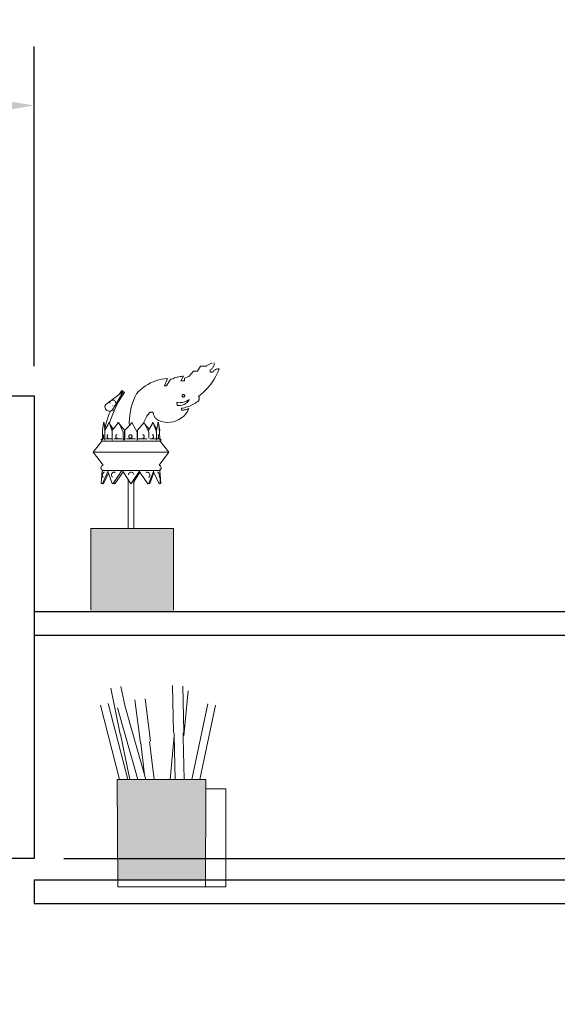
# Model space of a CAD drawing. Units: millimetres. Extents: x 7894 to 8038, y 6851 to 6951.
# Tile 8 of 49: x 7963 to 7975, y 6871 to 6892. Entities that reach past the tile are written whole.
import ezdxf

# ---------------------------------------------------------------- set-up
doc = ezdxf.new("R2010")
doc.units = ezdxf.units.MM
for name, color, linetype, lineweight in [('A-ANNO-DIMS', 2, 'Continuous', 18), ('A-FURN-ACCS', 8, 'Continuous', 13), ('A-FURN-CASE', 7, 'Continuous', 30), ('A-FURN-SHLF', 7, 'Continuous', 30)]:
    doc.layers.add(name, color=color, linetype=linetype, lineweight=lineweight)
doc.layers.add('A-FURN-ACCS-PATT', color=116, linetype='Continuous', lineweight=9, true_color=0x136734)
doc.styles.get("Standard").update_dxf_attribs({"font": 'arial.ttf'})
doc.dimstyles.new('ISO-25', dxfattribs={"dimtxt": 1, "dimasz": 1, "dimexe": 1.25, "dimexo": 0.625, "dimtad": 1, "dimdec": 0, "dimlunit": 4, "dimtxsty": 'Standard', "dimcen": 2.5, "dimclrt": 1, "dimadec": 0, "dimazin": 0, "dimtfac": 1, "dimtdec": 0, "dimtmove": 0, "dimatfit": 3, "dimfxl": 1, "dimarcsym": 0})

# ---------------------------------------------------------------- blocks, each defined once
blk = doc.blocks.new('DISPLAY-LEAF-FINIAL')
for p, q in [((2.209, 3.334), (2.276, 3.441)), ((2.276, 3.441), (2.398, 3.441)), ((2.398, 3.441), (2.409, 3.452)), ((2.409, 3.452), (2.421, 3.461)), ((2.421, 3.461), (2.434, 3.47)), ((2.434, 3.47), (2.447, 3.478)), ((2.447, 3.478), (2.461, 3.485)), ((2.461, 3.485), (2.475, 3.491)), ((2.475, 3.491), (2.489, 3.496)), ((2.493, 3.371), (2.48, 3.364)), ((2.48, 3.364), (2.48, 3.316)), ((2.489, 3.496), (2.504, 3.501)), ((2.505, 3.379), (2.493, 3.371)), ((2.504, 3.501), (2.519, 3.504)), ((2.516, 3.389), (2.505, 3.379)), ((2.527, 3.4), (2.516, 3.389)), ((2.536, 3.411), (2.527, 3.4)), ((2.544, 3.424), (2.536, 3.411)), ((2.54, 3.327), (2.549, 3.338)), ((2.551, 3.437), (2.544, 3.424)), ((2.549, 3.338), (2.558, 3.347)), ((2.556, 3.45), (2.551, 3.437)), ((2.56, 3.465), (2.556, 3.45)), ((2.558, 3.347), (2.569, 3.356)), ((2.563, 3.479), (2.56, 3.465)), ((2.565, 3.494), (2.563, 3.479)), ((2.565, 3.508), (2.565, 3.494)), ((2.569, 3.356), (2.58, 3.363)), ((2.58, 3.363), (2.592, 3.37)), ((2.592, 3.37), (2.604, 3.375)), ((2.604, 3.375), (2.617, 3.379)), ((2.617, 3.379), (2.63, 3.382)), ((2.63, 3.382), (2.643, 3.383)), ((2.643, 3.383), (2.657, 3.383)), ((2.67, 3.382), (2.646, 3.325)), ((2.657, 3.383), (2.67, 3.382)), ((1.27, 3.111), (1.328, 3.133)), ((1.328, 3.133), (1.388, 3.15)), ((1.388, 3.15), (1.449, 3.164)), ((1.449, 3.164), (1.51, 3.173)), ((1.51, 3.173), (1.572, 3.179)), ((1.572, 3.179), (1.511, 3.024)), ((1.55, 3.024), (1.632, 3.152)), ((1.632, 3.152), (1.654, 3.163)), ((1.654, 3.163), (1.676, 3.173)), ((1.676, 3.173), (1.699, 3.182)), ((1.699, 3.182), (1.722, 3.191)), ((1.722, 3.191), (1.745, 3.198)), ((1.745, 3.198), (1.769, 3.205)), ((1.769, 3.205), (1.793, 3.211)), ((1.793, 3.211), (1.817, 3.216)), ((1.817, 3.216), (1.841, 3.22)), ((1.841, 3.22), (1.865, 3.223)), ((1.914, 3.227), (1.854, 3.133)), ((1.854, 3.133), (1.934, 3.133)), ((1.865, 3.223), (1.889, 3.226)), ((1.889, 3.226), (1.914, 3.227)), ((1.934, 3.185), (2.023, 3.221)), ((1.934, 3.133), (1.934, 3.185)), ((2.023, 3.221), (2.127, 3.334)), ((2.127, 3.334), (2.209, 3.334)), ((2.48, 3.316), (2.533, 3.316)), ((2.56, 3.163), (2.527, 3.112)), ((2.533, 3.316), (2.54, 3.327)), ((2.591, 3.216), (2.56, 3.163)), ((2.62, 3.27), (2.591, 3.216)), ((2.646, 3.325), (2.62, 3.27)), ((0.605, 2.924), (0.547, 2.84)), ((0.634, 2.905), (0.605, 2.924)), ((0.962, 2.903), (1.007, 2.946)), ((1.007, 2.946), (1.055, 2.986)), ((1.055, 2.986), (1.105, 3.023)), ((1.105, 3.023), (1.158, 3.056)), ((1.158, 3.056), (1.213, 3.085)), ((1.213, 3.085), (1.27, 3.111)), ((1.511, 3.024), (1.55, 3.024)), ((2.371, 2.923), (2.327, 2.88)), ((2.413, 2.967), (2.371, 2.923)), ((2.453, 3.014), (2.413, 2.967)), ((2.491, 3.062), (2.453, 3.014)), ((2.527, 3.112), (2.491, 3.062)), ((0.379, 2.713), (0.264, 2.627)), ((0.367, 2.703), (0.379, 2.713)), ((0.547, 2.84), (0.379, 2.713)), ((0.379, 2.713), (0.393, 2.72)), ((0.393, 2.72), (0.409, 2.723)), ((0.409, 2.723), (0.425, 2.722)), ((0.425, 2.722), (0.44, 2.718)), ((0.44, 2.718), (0.453, 2.709)), ((0.634, 2.9), (0.463, 2.609)), ((0.541, 2.696), (0.599, 2.791)), ((0.634, 2.905), (0.547, 2.84)), ((0.599, 2.791), (0.663, 2.885)), ((0.634, 2.9), (0.634, 2.905)), ((0.663, 2.885), (0.634, 2.905)), ((0.853, 2.713), (0.826, 2.638)), ((0.884, 2.786), (0.853, 2.713)), ((0.92, 2.857), (0.884, 2.786)), ((0.92, 2.857), (0.962, 2.903)), ((1.883, 2.817), (1.885, 2.824)), ((1.883, 2.81), (1.883, 2.817)), ((1.885, 2.803), (1.883, 2.81)), ((1.885, 2.824), (1.889, 2.831)), ((1.888, 2.797), (1.885, 2.803)), ((1.894, 2.791), (1.888, 2.797)), ((1.889, 2.831), (1.894, 2.836)), ((1.894, 2.836), (1.9, 2.839)), ((1.9, 2.788), (1.894, 2.791)), ((1.9, 2.839), (1.907, 2.841)), ((1.907, 2.786), (1.9, 2.788)), ((1.907, 2.841), (1.914, 2.841)), ((1.914, 2.786), (1.907, 2.786)), ((1.914, 2.841), (1.921, 2.839)), ((1.921, 2.788), (1.914, 2.786)), ((1.921, 2.839), (1.928, 2.836)), ((1.928, 2.791), (1.921, 2.788)), ((1.928, 2.836), (1.933, 2.83)), ((1.933, 2.796), (1.928, 2.791)), ((1.933, 2.83), (1.937, 2.824)), ((1.936, 2.803), (1.933, 2.796)), ((1.938, 2.81), (1.936, 2.803)), ((1.937, 2.824), (1.938, 2.817)), ((1.938, 2.817), (1.938, 2.81)), ((2.017, 2.722), (1.996, 2.711)), ((2.023, 2.712), (2.007, 2.692)), ((2.036, 2.734), (2.017, 2.722)), ((2.036, 2.734), (2.023, 2.712)), ((2.235, 2.717), (2.23, 2.709)), ((2.281, 2.839), (2.233, 2.801)), ((2.233, 2.801), (2.238, 2.792)), ((2.24, 2.726), (2.235, 2.717)), ((2.238, 2.792), (2.242, 2.783)), ((2.243, 2.735), (2.24, 2.726)), ((2.242, 2.783), (2.245, 2.774)), ((2.245, 2.745), (2.243, 2.735)), ((2.245, 2.774), (2.246, 2.764)), ((2.246, 2.754), (2.245, 2.745)), ((2.246, 2.764), (2.246, 2.754)), ((2.327, 2.88), (2.281, 2.839)), ((0.253, 2.607), (0.249, 2.584)), ((0.249, 2.58), (0.249, 2.584)), ((0.249, 2.58), (0.251, 2.557)), ((0.251, 2.557), (0.259, 2.536)), ((0.264, 2.627), (0.253, 2.607)), ((0.259, 2.536), (0.272, 2.517)), ((0.272, 2.517), (0.29, 2.502)), ((0.353, 2.675), (0.358, 2.69)), ((0.353, 2.66), (0.353, 2.675)), ((0.353, 2.659), (0.353, 2.66)), ((0.353, 2.657), (0.353, 2.659)), ((0.358, 2.69), (0.367, 2.703)), ((0.38, 2.497), (0.4, 2.51)), ((0.398, 2.513), (0.402, 2.512)), ((0.403, 2.513), (0.4, 2.514)), ((0.4, 2.51), (0.402, 2.512)), ((0.402, 2.512), (0.403, 2.513)), ((0.402, 2.512), (0.44, 2.495)), ((0.403, 2.513), (0.415, 2.527)), ((0.403, 2.513), (0.44, 2.496)), ((0.409, 2.511), (0.408, 2.509)), ((0.42, 2.535), (0.409, 2.511)), ((0.414, 2.606), (0.413, 2.603)), ((0.461, 2.605), (0.415, 2.527)), ((0.44, 2.496), (0.486, 2.593)), ((0.443, 2.613), (0.446, 2.612)), ((0.451, 2.615), (0.449, 2.616)), ((0.453, 2.709), (0.464, 2.698)), ((0.463, 2.609), (0.461, 2.605)), ((0.486, 2.593), (0.461, 2.605)), ((0.463, 2.609), (0.488, 2.597)), ((0.464, 2.698), (0.471, 2.684)), ((0.471, 2.684), (0.475, 2.669)), ((0.474, 2.667), (0.475, 2.669)), ((0.474, 2.667), (0.475, 2.666)), ((0.541, 2.696), (0.488, 2.597)), ((0.804, 2.562), (0.787, 2.485)), ((0.826, 2.638), (0.804, 2.562)), ((1.793, 2.668), (1.77, 2.67)), ((1.77, 2.67), (1.776, 2.611)), ((1.801, 2.608), (1.776, 2.611)), ((1.816, 2.667), (1.793, 2.668)), ((1.827, 2.607), (1.801, 2.608)), ((1.84, 2.668), (1.816, 2.667)), ((1.852, 2.609), (1.827, 2.607)), ((1.863, 2.67), (1.84, 2.668)), ((1.878, 2.613), (1.852, 2.609)), ((1.886, 2.673), (1.863, 2.67)), ((1.903, 2.554), (1.872, 2.548)), ((1.872, 2.548), (1.872, 2.508)), ((1.872, 2.508), (1.885, 2.509)), ((1.902, 2.62), (1.878, 2.613)), ((1.885, 2.509), (1.898, 2.51)), ((1.909, 2.678), (1.886, 2.673)), ((1.898, 2.51), (1.911, 2.511)), ((1.926, 2.63), (1.902, 2.62)), ((1.934, 2.561), (1.903, 2.554)), ((1.931, 2.684), (1.909, 2.678)), ((1.911, 2.511), (1.924, 2.513)), ((1.924, 2.513), (1.937, 2.515)), ((1.949, 2.642), (1.926, 2.63)), ((1.954, 2.692), (1.931, 2.684)), ((1.964, 2.569), (1.934, 2.561)), ((1.937, 2.515), (1.95, 2.518)), ((1.97, 2.657), (1.949, 2.642)), ((1.95, 2.518), (1.963, 2.521)), ((1.975, 2.701), (1.954, 2.692)), ((1.963, 2.521), (1.976, 2.524)), ((1.994, 2.578), (1.964, 2.569)), ((1.99, 2.673), (1.97, 2.657)), ((1.996, 2.711), (1.975, 2.701)), ((1.976, 2.524), (1.988, 2.528)), ((1.988, 2.528), (2.001, 2.532)), ((2.007, 2.692), (1.99, 2.673)), ((2.024, 2.588), (1.994, 2.578)), ((2.026, 2.541), (1.997, 2.484)), ((2.001, 2.532), (2.013, 2.536)), ((2.013, 2.536), (2.026, 2.541)), ((2.053, 2.6), (2.024, 2.588)), ((2.082, 2.613), (2.053, 2.6)), ((2.11, 2.627), (2.082, 2.613)), ((2.137, 2.643), (2.11, 2.627)), ((2.164, 2.659), (2.137, 2.643)), ((2.19, 2.677), (2.164, 2.659)), ((2.216, 2.695), (2.19, 2.677)), ((2.223, 2.702), (2.216, 2.695)), ((2.23, 2.709), (2.223, 2.702)), ((0.295, 2.306), (0.263, 2.194)), ((0.29, 2.502), (0.311, 2.492)), ((0.332, 2.415), (0.295, 2.306)), ((0.311, 2.492), (0.334, 2.488)), ((0.363, 2.491), (0.332, 2.415)), ((0.334, 2.488), (0.358, 2.489)), ((0.358, 2.489), (0.363, 2.491)), ((0.361, 2.285), (0.398, 2.391)), ((0.363, 2.491), (0.38, 2.497)), ((0.365, 2.496), (0.363, 2.491)), ((0.398, 2.391), (0.44, 2.495)), ((0.766, 2.327), (0.763, 2.248)), ((0.774, 2.406), (0.766, 2.327)), ((0.787, 2.485), (0.774, 2.406)), ((1.092, 2.297), (1.075, 2.254)), ((1.113, 2.339), (1.092, 2.297)), ((1.136, 2.379), (1.113, 2.339)), ((1.163, 2.417), (1.136, 2.379)), ((1.193, 2.452), (1.163, 2.417)), ((1.198, 2.457), (1.193, 2.452)), ((1.204, 2.462), (1.198, 2.457)), ((1.211, 2.465), (1.204, 2.462)), ((1.218, 2.467), (1.211, 2.465)), ((1.225, 2.469), (1.218, 2.467)), ((1.232, 2.47), (1.225, 2.469)), ((1.239, 2.469), (1.232, 2.47)), ((1.247, 2.467), (1.239, 2.469)), ((1.254, 2.465), (1.247, 2.467)), ((1.26, 2.462), (1.254, 2.465)), ((1.266, 2.457), (1.26, 2.462)), ((1.271, 2.452), (1.266, 2.457)), ((1.274, 2.435), (1.271, 2.452)), ((1.278, 2.418), (1.274, 2.435)), ((1.283, 2.402), (1.278, 2.418)), ((1.29, 2.386), (1.283, 2.402)), ((1.298, 2.371), (1.29, 2.386)), ((1.308, 2.357), (1.298, 2.371)), ((1.319, 2.343), (1.308, 2.357)), ((1.331, 2.331), (1.319, 2.343)), ((1.343, 2.319), (1.331, 2.331)), ((1.357, 2.309), (1.343, 2.319)), ((1.372, 2.3), (1.357, 2.309)), ((1.387, 2.292), (1.372, 2.3)), ((1.816, 2.31), (1.759, 2.283)), ((1.87, 2.344), (1.816, 2.31)), ((1.918, 2.385), (1.87, 2.344)), ((1.961, 2.432), (1.918, 2.385)), ((1.997, 2.484), (1.961, 2.432)), ((0.213, 2.19), (0.195, 2.086)), ((0.195, 2.086), (0.195, 2.048)), ((0.213, 2.19), (0.215, 2.201)), ((0.215, 2.201), (0.22, 2.245)), ((0.223, 2.245), (0.215, 2.201)), ((0.223, 2.245), (0.22, 2.245)), ((0.223, 2.245), (0.23, 2.245)), ((0.232, 2.22), (0.23, 2.245)), ((0.232, 2.22), (0.25, 2.138)), ((0.244, 2.11), (0.232, 2.22)), ((0.244, 2.11), (0.239, 2.089)), ((0.25, 2.138), (0.244, 2.11)), ((0.248, 2.065), (0.244, 2.11)), ((0.317, 2.207), (0.248, 2.086)), ((0.248, 2.086), (0.248, 2.065)), ((0.263, 2.194), (0.25, 2.138)), ((0.25, 2.138), (0.256, 2.115)), ((0.297, 2.185), (0.292, 2.162)), ((0.317, 2.207), (0.33, 2.245)), ((0.338, 2.245), (0.317, 2.207)), ((0.332, 2.245), (0.33, 2.245)), ((0.344, 2.245), (0.338, 2.245)), ((0.347, 2.235), (0.344, 2.245)), ((0.347, 2.235), (0.361, 2.285)), ((0.354, 2.213), (0.347, 2.235)), ((0.354, 2.213), (0.42, 2.104)), ((0.404, 2.061), (0.354, 2.213)), ((0.42, 2.104), (0.404, 2.086)), ((0.404, 2.086), (0.404, 2.061)), ((0.507, 2.209), (0.42, 2.104)), ((0.507, 2.209), (0.525, 2.245)), ((0.532, 2.239), (0.507, 2.209)), ((0.528, 2.245), (0.525, 2.245)), ((0.528, 2.245), (0.532, 2.239)), ((0.537, 2.245), (0.532, 2.239)), ((0.54, 2.245), (0.537, 2.245)), ((0.556, 2.211), (0.54, 2.245)), ((0.548, 2.22), (0.556, 2.211)), ((0.556, 2.211), (0.663, 2.086)), ((0.636, 2.045), (0.556, 2.211)), ((0.663, 2.086), (0.663, 1.903)), ((0.765, 2.186), (0.671, 2.086)), ((0.671, 2.086), (0.671, 1.903)), ((0.763, 2.248), (0.765, 2.186)), ((0.821, 2.245), (0.765, 2.186)), ((0.93, 2.045), (0.821, 2.245)), ((1.07, 2.239), (0.939, 2.086)), ((0.939, 2.086), (0.939, 1.934)), ((1.07, 2.239), (1.069, 2.235)), ((1.071, 2.24), (1.07, 2.239)), ((1.07, 2.239), (1.071, 2.237)), ((1.075, 2.254), (1.071, 2.24)), ((1.074, 2.245), (1.071, 2.24)), ((1.074, 2.245), (1.078, 2.245)), ((1.095, 2.209), (1.078, 2.245)), ((1.095, 2.209), (1.182, 2.104)), ((1.095, 2.209), (1.171, 2.054)), ((1.182, 2.104), (1.171, 2.086)), ((1.171, 2.086), (1.171, 2.054)), ((1.248, 2.213), (1.182, 2.104)), ((1.248, 2.213), (1.258, 2.245)), ((1.265, 2.242), (1.248, 2.213)), ((1.258, 2.245), (1.264, 2.245)), ((1.264, 2.245), (1.265, 2.242)), ((1.267, 2.245), (1.265, 2.242)), ((1.267, 2.245), (1.272, 2.245)), ((1.285, 2.207), (1.272, 2.245)), ((1.285, 2.207), (1.344, 2.103)), ((1.285, 2.207), (1.34, 2.048)), ((1.344, 2.103), (1.34, 2.086)), ((1.34, 2.086), (1.34, 2.048)), ((1.37, 2.22), (1.344, 2.103)), ((1.37, 2.22), (1.372, 2.245)), ((1.375, 2.245), (1.37, 2.22)), ((1.372, 2.245), (1.375, 2.245)), ((1.375, 2.245), (1.382, 2.245)), ((1.382, 2.245), (1.389, 2.19)), ((1.447, 2.27), (1.387, 2.292)), ((1.389, 2.19), (1.408, 2.086)), ((1.407, 2.045), (1.389, 2.19)), ((1.408, 2.086), (1.407, 2.045)), ((1.509, 2.256), (1.447, 2.27)), ((1.572, 2.25), (1.509, 2.256)), ((1.635, 2.253), (1.572, 2.25)), ((1.698, 2.264), (1.635, 2.253)), ((1.759, 2.283), (1.698, 2.264)), ((0.17, 1.877), (0.172, 1.885)), ((0.17, 1.87), (0.17, 1.877)), ((0.172, 1.885), (0.176, 1.892)), ((0.176, 1.892), (0.182, 1.898)), ((0.182, 1.898), (0.189, 1.901)), ((0.189, 1.901), (0.195, 1.903)), ((0.195, 2.045), (0.195, 2.048)), ((0.195, 2.045), (0.195, 1.903)), ((0.195, 1.903), (0.195, 1.901)), ((0.195, 1.903), (0.196, 1.903)), ((0.195, 1.898), (0.195, 1.87)), ((0.196, 1.903), (0.198, 1.903)), ((0.196, 1.903), (0.197, 1.903)), ((0.237, 1.903), (0.198, 1.903)), ((0.207, 1.965), (0.208, 1.973)), ((0.207, 1.956), (0.207, 1.965)), ((0.207, 1.947), (0.207, 1.956)), ((0.207, 1.938), (0.207, 1.947)), ((0.208, 1.93), (0.207, 1.938)), ((0.208, 1.973), (0.209, 1.979)), ((0.209, 1.924), (0.208, 1.93)), ((0.209, 1.979), (0.211, 1.984)), ((0.211, 1.919), (0.209, 1.924)), ((0.21, 1.956), (0.211, 1.965)), ((0.21, 1.947), (0.21, 1.956)), ((0.211, 1.938), (0.21, 1.947)), ((0.211, 1.984), (0.213, 1.986)), ((0.211, 1.965), (0.212, 1.973)), ((0.212, 1.93), (0.211, 1.938)), ((0.213, 1.917), (0.211, 1.919)), ((0.212, 1.973), (0.213, 1.979)), ((0.213, 1.924), (0.212, 1.93)), ((0.216, 1.986), (0.213, 1.986)), ((0.213, 1.979), (0.214, 1.984)), ((0.216, 1.947), (0.213, 1.924)), ((0.214, 1.919), (0.213, 1.924)), ((0.214, 1.917), (0.213, 1.917)), ((0.214, 1.984), (0.216, 1.986)), ((0.216, 1.917), (0.214, 1.919)), ((0.216, 1.917), (0.214, 1.917)), ((0.217, 1.965), (0.216, 1.956)), ((0.216, 1.956), (0.216, 1.947)), ((0.216, 1.947), (0.217, 1.938)), ((0.218, 1.917), (0.216, 1.917)), ((0.218, 1.973), (0.217, 1.965)), ((0.218, 1.967), (0.217, 1.965)), ((0.217, 1.938), (0.218, 1.93)), ((0.219, 1.979), (0.218, 1.973)), ((0.218, 1.973), (0.218, 1.967)), ((0.218, 1.93), (0.219, 1.924)), ((0.22, 1.981), (0.219, 1.979)), ((0.22, 1.981), (0.219, 1.979)), ((0.219, 1.924), (0.22, 1.921)), ((0.221, 1.973), (0.22, 1.965)), ((0.22, 1.965), (0.22, 1.956)), ((0.22, 1.956), (0.22, 1.947)), ((0.22, 1.947), (0.22, 1.938)), ((0.22, 1.938), (0.221, 1.93)), ((0.222, 1.975), (0.221, 1.973)), ((0.221, 1.93), (0.222, 1.928)), ((0.248, 1.903), (0.244, 1.903)), ((0.245, 1.898), (0.244, 1.886)), ((0.248, 1.897), (0.244, 1.897)), ((0.248, 1.925), (0.246, 1.901)), ((0.248, 2.065), (0.248, 1.903)), ((0.248, 1.903), (0.248, 1.901)), ((0.248, 1.898), (0.248, 1.897)), ((0.248, 1.897), (0.248, 1.87)), ((0.391, 1.903), (0.265, 1.903)), ((0.295, 1.956), (0.297, 1.965)), ((0.295, 1.947), (0.295, 1.956)), ((0.297, 1.938), (0.295, 1.947)), ((0.297, 1.965), (0.3, 1.973)), ((0.3, 1.93), (0.297, 1.938)), ((0.3, 1.973), (0.304, 1.979)), ((0.303, 1.924), (0.3, 1.93)), ((0.308, 1.919), (0.303, 1.924)), ((0.304, 1.979), (0.308, 1.984)), ((0.308, 1.984), (0.314, 1.986)), ((0.313, 1.917), (0.308, 1.919)), ((0.319, 1.917), (0.313, 1.917)), ((0.316, 1.986), (0.314, 1.986)), ((0.322, 1.917), (0.319, 1.917)), ((0.404, 2.061), (0.404, 1.901)), ((0.404, 1.898), (0.404, 1.87)), ((0.439, 1.903), (0.607, 1.903)), ((0.476, 1.956), (0.478, 1.965)), ((0.476, 1.947), (0.476, 1.956)), ((0.478, 1.938), (0.476, 1.947)), ((0.478, 1.965), (0.482, 1.973)), ((0.482, 1.93), (0.478, 1.938)), ((0.482, 1.973), (0.488, 1.979)), ((0.488, 1.924), (0.482, 1.93)), ((0.488, 1.979), (0.495, 1.984)), ((0.495, 1.919), (0.488, 1.924)), ((0.495, 1.984), (0.502, 1.986)), ((0.502, 1.917), (0.495, 1.919)), ((0.504, 1.986), (0.502, 1.986)), ((0.51, 1.917), (0.502, 1.917)), ((0.512, 1.917), (0.51, 1.917)), ((0.637, 1.903), (0.634, 1.903)), ((0.637, 1.897), (0.634, 1.897)), ((0.636, 2.045), (0.637, 1.903)), ((0.637, 1.903), (0.637, 1.901)), ((0.663, 1.903), (0.637, 1.903)), ((0.637, 1.898), (0.637, 1.897)), ((0.637, 1.897), (0.637, 1.87)), ((0.663, 1.897), (0.637, 1.897)), ((0.663, 1.903), (0.671, 1.903)), ((0.663, 1.903), (0.663, 1.901)), ((0.663, 1.898), (0.663, 1.897)), ((0.663, 1.897), (0.663, 1.87)), ((0.671, 1.897), (0.663, 1.897)), ((0.671, 1.903), (0.671, 1.901)), ((0.671, 1.898), (0.671, 1.897)), ((0.671, 1.897), (0.671, 1.87)), ((0.708, 1.903), (0.894, 1.903)), ((0.754, 1.956), (0.756, 1.965)), ((0.754, 1.947), (0.754, 1.956)), ((0.756, 1.938), (0.754, 1.947)), ((0.756, 1.965), (0.761, 1.973)), ((0.761, 1.93), (0.756, 1.938)), ((0.761, 1.973), (0.767, 1.979)), ((0.767, 1.924), (0.761, 1.93)), ((0.767, 1.979), (0.775, 1.984)), ((0.775, 1.919), (0.767, 1.924)), ((0.775, 1.984), (0.784, 1.986)), ((0.784, 1.917), (0.775, 1.919)), ((0.784, 1.986), (0.793, 1.986)), ((0.793, 1.917), (0.784, 1.917)), ((0.793, 1.986), (0.802, 1.984)), ((0.802, 1.919), (0.793, 1.917)), ((0.802, 1.984), (0.81, 1.979)), ((0.81, 1.924), (0.802, 1.919)), ((0.81, 1.979), (0.816, 1.973)), ((0.816, 1.93), (0.81, 1.924)), ((0.816, 1.973), (0.821, 1.965)), ((0.821, 1.938), (0.816, 1.93)), ((0.821, 1.965), (0.823, 1.956)), ((0.823, 1.947), (0.821, 1.938)), ((0.823, 1.956), (0.823, 1.947)), ((0.93, 2.045), (0.931, 1.934)), ((0.939, 1.934), (0.931, 1.934)), ((0.931, 1.934), (0.931, 1.903)), ((0.931, 1.903), (0.931, 1.901)), ((0.939, 1.903), (0.931, 1.903)), ((0.931, 1.898), (0.931, 1.897)), ((0.931, 1.897), (0.932, 1.87)), ((0.939, 1.897), (0.931, 1.897)), ((0.942, 1.934), (0.939, 1.934)), ((0.939, 1.934), (0.939, 1.903)), ((0.942, 1.903), (0.939, 1.903)), ((0.939, 1.903), (0.939, 1.901)), ((0.939, 1.898), (0.939, 1.897)), ((0.942, 1.897), (0.939, 1.897)), ((0.939, 1.897), (0.939, 1.87)), ((0.953, 1.903), (1.146, 1.903)), ((1.022, 1.935), (1.021, 1.935)), ((1.044, 1.986), (1.046, 1.986)), ((1.046, 1.986), (1.054, 1.986)), ((1.052, 1.917), (1.054, 1.917)), ((1.054, 1.986), (1.062, 1.984)), ((1.062, 1.919), (1.054, 1.917)), ((1.062, 1.984), (1.069, 1.979)), ((1.069, 1.924), (1.062, 1.919)), ((1.069, 1.979), (1.075, 1.973)), ((1.075, 1.93), (1.069, 1.924)), ((1.075, 1.973), (1.079, 1.965)), ((1.079, 1.938), (1.075, 1.93)), ((1.079, 1.965), (1.081, 1.956)), ((1.081, 1.947), (1.079, 1.938)), ((1.081, 1.956), (1.081, 1.947)), ((1.176, 2.045), (1.171, 2.054)), ((1.176, 2.045), (1.177, 1.914)), ((1.33, 1.903), (1.197, 1.903)), ((1.249, 1.986), (1.251, 1.986)), ((1.251, 1.986), (1.257, 1.986)), ((1.254, 1.917), (1.257, 1.917)), ((1.257, 1.986), (1.263, 1.984)), ((1.263, 1.919), (1.257, 1.917)), ((1.263, 1.984), (1.268, 1.979)), ((1.268, 1.924), (1.263, 1.919)), ((1.268, 1.979), (1.272, 1.973)), ((1.272, 1.93), (1.268, 1.924)), ((1.272, 1.973), (1.275, 1.965)), ((1.275, 1.938), (1.272, 1.93)), ((1.275, 1.965), (1.276, 1.956)), ((1.276, 1.947), (1.275, 1.938)), ((1.276, 1.956), (1.276, 1.947)), ((1.341, 2.045), (1.34, 2.048)), ((1.341, 2.045), (1.342, 1.903)), ((1.347, 1.903), (1.342, 1.903)), ((1.342, 1.903), (1.342, 1.901)), ((1.342, 1.898), (1.342, 1.897)), ((1.347, 1.897), (1.342, 1.897)), ((1.342, 1.897), (1.342, 1.87)), ((1.356, 1.903), (1.4, 1.903)), ((1.373, 1.986), (1.376, 1.986)), ((1.378, 1.919), (1.375, 1.917)), ((1.375, 1.917), (1.379, 1.917)), ((1.376, 1.986), (1.378, 1.984)), ((1.376, 1.986), (1.377, 1.986)), ((1.377, 1.986), (1.379, 1.986)), ((1.378, 1.984), (1.379, 1.979)), ((1.379, 1.924), (1.378, 1.919)), ((1.379, 1.986), (1.381, 1.984)), ((1.379, 1.979), (1.381, 1.973)), ((1.381, 1.93), (1.379, 1.924)), ((1.381, 1.919), (1.379, 1.917)), ((1.381, 1.984), (1.383, 1.979)), ((1.381, 1.973), (1.382, 1.965)), ((1.382, 1.938), (1.381, 1.93)), ((1.383, 1.924), (1.381, 1.919)), ((1.382, 1.965), (1.382, 1.956)), ((1.382, 1.956), (1.382, 1.947)), ((1.382, 1.947), (1.382, 1.938)), ((1.383, 1.979), (1.384, 1.973)), ((1.384, 1.93), (1.383, 1.924)), ((1.384, 1.973), (1.385, 1.965)), ((1.385, 1.938), (1.384, 1.93)), ((1.385, 1.965), (1.386, 1.956)), ((1.386, 1.947), (1.385, 1.938)), ((1.386, 1.956), (1.386, 1.947)), ((1.407, 2.045), (1.408, 1.903)), ((1.408, 1.903), (1.413, 1.901)), ((1.408, 1.903), (1.408, 1.901)), ((1.408, 1.898), (1.408, 1.87)), ((1.413, 1.901), (1.42, 1.898)), ((1.42, 1.898), (1.426, 1.892)), ((1.426, 1.892), (1.43, 1.885)), ((1.43, 1.885), (1.432, 1.877)), ((1.432, 1.877), (1.433, 1.87)), ((0, 1.62), (0.181, 1.849)), ((0.172, 1.862), (0.17, 1.87)), ((0.175, 1.855), (0.172, 1.862)), ((0.181, 1.849), (0.175, 1.855)), ((0.195, 1.862), (0.195, 1.855)), ((0.195, 1.855), (0.195, 1.855)), ((0.205, 1.855), (0.195, 1.855)), ((0.205, 1.855), (0.205, 1.851)), ((0.248, 1.855), (0.205, 1.855)), ((0.205, 1.851), (0.205, 1.849)), ((0.24, 1.855), (0.24, 1.849)), ((0.248, 1.862), (0.248, 1.855)), ((0.248, 1.855), (0.276, 1.855)), ((0.275, 1.849), (0.276, 1.855)), ((0.276, 1.855), (0.405, 1.855)), ((0.404, 1.862), (0.405, 1.855)), ((0.405, 1.855), (0.637, 1.855)), ((0.637, 1.862), (0.637, 1.855)), ((0.663, 1.855), (0.637, 1.855)), ((0.663, 1.862), (0.663, 1.855)), ((0.671, 1.862), (0.671, 1.855)), ((0.671, 1.855), (0.932, 1.855)), ((0.932, 1.862), (0.932, 1.855)), ((0.939, 1.855), (0.932, 1.855)), ((0.939, 1.862), (0.939, 1.855)), ((1.342, 1.855), (0.939, 1.855)), ((1.342, 1.862), (1.342, 1.855)), ((1.408, 1.855), (1.342, 1.855)), ((1.408, 1.862), (1.408, 1.855)), ((1.427, 1.855), (1.421, 1.849)), ((1.421, 1.849), (1.602, 1.62)), ((1.431, 1.862), (1.427, 1.855)), ((1.433, 1.87), (1.431, 1.862)), ((0.207, 1.343), (0, 1.62)), ((1.602, 1.62), (0, 1.62)), ((1.602, 1.62), (1.395, 1.343)), ((0.164, 1.297), (0.168, 1.31)), ((0.164, 1.283), (0.164, 1.297)), ((0.167, 1.27), (0.164, 1.283)), ((0.173, 1.258), (0.167, 1.27)), ((0.168, 1.31), (0.174, 1.321)), ((0.182, 1.248), (0.173, 1.258)), ((0.174, 1.321), (0.183, 1.331)), ((0.183, 1.331), (0.195, 1.338)), ((0.195, 1.338), (0.207, 1.343)), ((1.395, 1.343), (1.408, 1.338)), ((1.408, 1.338), (1.419, 1.331)), ((1.419, 1.331), (1.428, 1.321)), ((1.429, 1.258), (1.42, 1.248)), ((1.428, 1.321), (1.434, 1.31)), ((1.435, 1.27), (1.429, 1.258)), ((1.434, 1.31), (1.438, 1.297)), ((1.438, 1.283), (1.435, 1.27)), ((1.438, 1.297), (1.438, 1.283)), ((0.171, 0.955), (0.191, 1.234)), ((0.193, 1.24), (0.182, 1.248)), ((0.219, 1.234), (0.191, 1.234)), ((0.206, 1.236), (0.193, 1.24)), ((0.194, 1.111), (0.196, 1.124)), ((0.195, 1.101), (0.194, 1.111)), ((0.196, 1.094), (0.195, 1.101)), ((0.196, 0.954), (0.311, 1.21)), ((0.196, 1.124), (0.198, 1.137)), ((0.199, 1.09), (0.196, 1.094)), ((0.198, 1.137), (0.202, 1.152)), ((0.203, 1.089), (0.199, 1.09)), ((0.202, 1.152), (0.206, 1.165)), ((0.204, 1.088), (0.203, 1.089)), ((0.219, 1.234), (0.206, 1.236)), ((0.206, 1.165), (0.212, 1.177)), ((0.211, 1.096), (0.213, 1.092)), ((0.212, 1.177), (0.217, 1.187)), ((0.213, 1.092), (0.214, 1.092)), ((0.214, 1.1), (0.214, 1.098)), ((0.215, 0.949), (0.324, 1.172)), ((0.217, 1.187), (0.223, 1.193)), ((0.219, 1.234), (0.297, 1.234)), ((0.223, 1.193), (0.228, 1.197)), ((0.228, 1.197), (0.232, 1.196)), ((0.232, 1.195), (0.232, 1.196)), ((0.232, 1.195), (0.237, 1.195)), ((0.297, 1.234), (0.302, 1.234)), ((0.303, 1.232), (0.297, 1.234)), ((0.303, 1.232), (0.302, 1.234)), ((0.302, 1.234), (0.594, 1.234)), ((0.311, 1.21), (0.303, 1.232)), ((0.324, 1.172), (0.311, 1.21)), ((0.402, 0.955), (0.324, 1.172)), ((0.387, 1.137), (0.389, 1.152)), ((0.387, 1.124), (0.387, 1.137)), ((0.391, 1.111), (0.387, 1.124)), ((0.389, 1.152), (0.395, 1.165)), ((0.397, 1.101), (0.391, 1.111)), ((0.395, 1.165), (0.403, 1.177)), ((0.406, 1.094), (0.397, 1.101)), ((0.403, 1.177), (0.413, 1.187)), ((0.409, 1.092), (0.406, 1.094)), ((0.413, 1.187), (0.424, 1.193)), ((0.424, 1.193), (0.436, 1.197)), ((0.434, 0.975), (0.609, 1.228)), ((0.436, 1.197), (0.448, 1.196)), ((0.448, 1.196), (0.458, 1.192)), ((0.455, 0.949), (0.632, 1.205)), ((0.458, 1.192), (0.461, 1.191)), ((0.594, 1.234), (0.617, 1.234)), ((0.609, 1.228), (0.594, 1.234)), ((0.617, 1.228), (0.617, 1.234)), ((0.952, 1.234), (0.617, 1.234)), ((0.632, 1.205), (0.617, 1.228)), ((0.742, 1.037), (0.632, 1.205)), ((0.747, 1.137), (0.748, 1.152)), ((0.747, 1.136), (0.747, 1.137)), ((0.748, 1.152), (0.752, 1.165)), ((0.752, 1.165), (0.76, 1.177)), ((0.76, 1.177), (0.77, 1.187)), ((0.77, 1.187), (0.783, 1.193)), ((0.783, 1.193), (0.797, 1.197)), ((0.797, 1.197), (0.812, 1.196)), ((0.812, 1.196), (0.826, 1.192)), ((0.826, 1.192), (0.838, 1.185)), ((0.838, 1.185), (0.848, 1.175)), ((0.848, 1.175), (0.855, 1.162)), ((0.855, 1.162), (0.859, 1.148)), ((0.859, 1.147), (0.859, 1.148)), ((0.86, 1.041), (0.977, 1.215)), ((0.86, 0.992), (0.99, 1.195)), ((0.86, 1.041), (0.86, 1.047)), ((0.981, 1.234), (0.952, 1.234)), ((0.977, 1.215), (0.974, 1.218)), ((0.99, 1.195), (0.977, 1.215)), ((0.981, 1.234), (0.982, 1.234)), ((0.982, 1.234), (0.983, 1.234)), ((1.284, 1.234), (0.983, 1.234)), ((1.16, 0.949), (0.99, 1.195)), ((1.124, 1.192), (1.126, 1.193)), ((1.126, 1.193), (1.127, 1.193)), ((1.127, 1.193), (1.138, 1.197)), ((1.138, 1.197), (1.15, 1.196)), ((1.15, 1.196), (1.162, 1.192)), ((1.162, 1.192), (1.174, 1.185)), ((1.174, 1.092), (1.172, 1.091)), ((1.174, 1.185), (1.184, 1.175)), ((1.174, 1.092), (1.175, 1.092)), ((1.185, 1.099), (1.175, 1.092)), ((1.177, 0.964), (1.275, 1.212)), ((1.184, 1.175), (1.191, 1.162)), ((1.192, 1.109), (1.185, 1.099)), ((1.191, 1.162), (1.196, 1.148)), ((1.196, 1.121), (1.192, 1.109)), ((1.196, 1.148), (1.198, 1.134)), ((1.198, 1.134), (1.196, 1.121)), ((1.202, 0.955), (1.285, 1.19)), ((1.275, 1.212), (1.283, 1.232)), ((1.285, 1.19), (1.275, 1.212)), ((1.283, 1.232), (1.29, 1.234)), ((1.283, 1.232), (1.284, 1.234)), ((1.284, 1.234), (1.29, 1.234)), ((1.398, 0.949), (1.285, 1.19)), ((1.29, 1.234), (1.383, 1.234)), ((1.359, 1.195), (1.364, 1.197)), ((1.359, 1.195), (1.362, 1.195)), ((1.364, 1.197), (1.369, 1.196)), ((1.369, 1.196), (1.374, 1.192)), ((1.374, 1.192), (1.38, 1.185)), ((1.38, 1.185), (1.386, 1.175)), ((1.397, 1.236), (1.383, 1.234)), ((1.41, 1.234), (1.383, 1.234)), ((1.386, 1.175), (1.392, 1.162)), ((1.392, 1.089), (1.39, 1.088)), ((1.39, 1.088), (1.395, 1.089)), ((1.392, 1.162), (1.396, 1.148)), ((1.399, 1.092), (1.395, 1.089)), ((1.396, 1.148), (1.4, 1.134)), ((1.409, 1.24), (1.397, 1.236)), ((1.401, 1.099), (1.399, 1.092)), ((1.4, 1.134), (1.402, 1.121)), ((1.402, 1.109), (1.401, 1.099)), ((1.402, 1.121), (1.402, 1.109)), ((1.42, 1.248), (1.409, 1.24)), ((1.411, 1.234), (1.41, 1.234)), ((1.411, 1.232), (1.411, 1.234)), ((1.435, 0.955), (1.411, 1.232)), ((1.42, 0.955), (1.411, 1.232)), ((0.194, 0.949), (0.171, 0.955)), ((0.194, 0.949), (0.196, 0.954)), ((0.215, 0.949), (0.196, 0.954)), ((0.416, 0.949), (0.402, 0.955)), ((0.416, 0.949), (0.434, 0.975)), ((0.442, 0.955), (0.434, 0.975)), ((0.455, 0.949), (0.442, 0.955)), ((0.742, 0), (0.742, 1.037)), ((0.799, 0.949), (0.742, 1.037)), ((0.799, 0.949), (0.816, 0.974)), ((0.816, 0.974), (0.814, 0.977)), ((0.816, 0.974), (0.86, 1.041)), ((0.816, 0.973), (0.816, 0.974)), ((0.843, 0.965), (0.86, 0.992)), ((0.86, 0.992), (0.86, 1.041)), ((0.86, 0), (0.86, 0.992)), ((1.16, 0.949), (1.173, 0.955)), ((1.173, 0.955), (1.177, 0.964)), ((1.187, 0.949), (1.177, 0.964)), ((1.187, 0.949), (1.202, 0.955)), ((1.398, 0.949), (1.41, 0.953)), ((1.41, 0.953), (1.42, 0.955)), ((1.412, 0.949), (1.41, 0.953)), ((1.412, 0.949), (1.435, 0.955))]:
    blk.add_line(p, q)
blk = doc.blocks.new('DISPLAY-REED-SPRAY')
for p, q in [((0.218, 1.934), (0.42, 0.963)), ((0.515, 1.573), (0.435, 1.972)), ((1.548, 0.994), (1.529, 1.989)), ((1.766, 1.01), (1.742, 1.98)), ((1.77, 0.926), (1.861, 1.878)), ((0.846, 0.767), (0.729, 1.689)), ((1.062, 0.811), (0.945, 1.707)), ((0, 1.572), (0.406, 0.001)), ((0.578, 0.003), (0.162, 1.611)), ((0.792, 0), (0.361, 1.519)), ((0.935, 0.103), (0.519, 1.567)), ((1.938, 0.003), (2.275, 1.603)), ((2.108, 0.001), (2.44, 1.573)), ((0.62, 0.003), (0.428, 0.96)), ((1.477, 0.003), (1.56, 0.927)), ((1.56, 0.991), (1.561, 0.935)), ((1.56, 0.927), (1.561, 0.935)), ((1.56, 0.927), (1.58, 0.003)), ((1.753, 0.892), (1.751, 0.999)), ((1.753, 0.892), (1.755, 0.914)), ((1.771, 0.003), (1.753, 0.892)), ((0.935, 0.103), (0.852, 0.78)), ((1.139, 0.003), (1.042, 0.808)), ((0.963, 0.002), (0.935, 0.103))]:
    blk.add_line(p, q)
blk = doc.blocks.new('*D36')
at = {"layer": 'A-ANNO-DIMS', "color": 0, "lineweight": -2, "transparency": 16777216}
for p, q in [((7980.836, 6877.959), (7980.836, 6858.512)), ((7944.487, 6864.436), (7944.487, 6858.512)), ((7945.487, 6859.762), (7979.836, 6859.762))]:
    blk.add_line(p, q, dxfattribs=at)
at = {"layer": 'A-ANNO-DIMS', "color": 0, "transparency": 16777216}
for points in [[(7945.487, 6859.929), (7945.487, 6859.596), (7944.487, 6859.762)], [(7979.836, 6859.929), (7979.836, 6859.596), (7980.836, 6859.762)]]:
    blk.add_solid(points, dxfattribs=at)
at = {"layer": 'Defpoints', "color": 0, "transparency": 16777216}
for p in [(7980.836, 6878.584), (7944.487, 6865.061), (7980.836, 6859.762)]:
    blk.add_point(p, dxfattribs=at)
at = {"layer": 'A-ANNO-DIMS', "color": 1, "transparency": 16777216, "insert": (7962.661, 6860.905), "char_height": 1, "attachment_point": 5}
blk.add_mtext('3\'-0 1/2"', dxfattribs=at)
blk = doc.blocks.new('*D39')
at = {"layer": 'A-ANNO-DIMS', "color": 0, "lineweight": -2, "transparency": 16777216}
for p, q in [((7982.683, 6874.858), (7982.683, 6879.766)), ((7964.157, 6873.858), (7983.933, 6873.858)), ((7982.683, 6872.903), (7982.683, 6873.858)), ((7981.461, 6872.903), (7983.933, 6872.903)), ((7982.683, 6871.903), (7982.683, 6870.903))]:
    blk.add_line(p, q, dxfattribs=at)
at = {"layer": 'A-ANNO-DIMS', "color": 0, "transparency": 16777216}
for points in [[(7982.517, 6874.858), (7982.85, 6874.858), (7982.683, 6873.858)], [(7982.517, 6871.903), (7982.85, 6871.903), (7982.683, 6872.903)]]:
    blk.add_solid(points, dxfattribs=at)
at = {"layer": 'Defpoints', "color": 0, "transparency": 16777216}
for p in [(7963.532, 6873.858), (7982.683, 6873.858), (7980.836, 6872.903)]:
    blk.add_point(p, dxfattribs=at)
at = {"layer": 'A-ANNO-DIMS', "color": 1, "transparency": 16777216, "insert": (7981.548, 6877.812), "char_height": 1, "attachment_point": 5, "rotation": 90}
blk.add_mtext('0\'-1"', dxfattribs=at)
blk = doc.blocks.new('*D40')
at = {"layer": 'A-ANNO-DIMS', "color": 0, "lineweight": -2, "transparency": 16777216}
for p, q in [((7982.683, 6878.584), (7982.683, 6885.822)), ((7981.461, 6878.584), (7983.933, 6878.584)), ((7982.683, 6874.858), (7982.683, 6877.584)), ((7964.157, 6873.858), (7983.933, 6873.858))]:
    blk.add_line(p, q, dxfattribs=at)
at = {"layer": 'A-ANNO-DIMS', "color": 0, "transparency": 16777216}
for points in [[(7982.517, 6877.584), (7982.85, 6877.584), (7982.683, 6878.584)], [(7982.517, 6874.858), (7982.85, 6874.858), (7982.683, 6873.858)]]:
    blk.add_solid(points, dxfattribs=at)
at = {"layer": 'Defpoints', "color": 0, "transparency": 16777216}
for p in [(7980.836, 6878.584), (7982.683, 6878.584), (7963.532, 6873.858)]:
    blk.add_point(p, dxfattribs=at)
at = {"layer": 'A-ANNO-DIMS', "color": 1, "transparency": 16777216, "insert": (7981.541, 6882.703), "char_height": 1, "attachment_point": 5, "rotation": 90}
blk.add_mtext('0\'-4 1/2"', dxfattribs=at)
blk = doc.blocks.new('*D43')
at = {"layer": 'A-ANNO-DIMS', "color": 0, "lineweight": -2, "transparency": 16777216}
for p, q in [((7955.37, 6888.006), (7955.37, 6891.056)), ((7963.532, 6884.283), (7963.532, 6891.056)), ((7956.37, 6889.806), (7962.532, 6889.806))]:
    blk.add_line(p, q, dxfattribs=at)
at = {"layer": 'A-ANNO-DIMS', "color": 0, "transparency": 16777216}
for points in [[(7956.37, 6889.972), (7956.37, 6889.639), (7955.37, 6889.806)], [(7962.532, 6889.972), (7962.532, 6889.639), (7963.532, 6889.806)]]:
    blk.add_solid(points, dxfattribs=at)
at = {"layer": 'Defpoints', "color": 0, "transparency": 16777216}
for p in [(7963.532, 6889.806), (7955.37, 6887.381), (7963.532, 6883.658)]:
    blk.add_point(p, dxfattribs=at)
at = {"layer": 'A-ANNO-DIMS', "color": 1, "transparency": 16777216, "insert": (7959.451, 6890.941), "char_height": 1, "attachment_point": 5}
blk.add_mtext('0\'-8"', dxfattribs=at)

msp = doc.modelspace()

# ---------------------------------------------------------------- hatches: boundary and pattern name
at = {"layer": 'A-FURN-ACCS-PATT'}
h = msp.add_hatch(color=256, dxfattribs=at)
h.dxf.hatch_style = 1
h.paths.add_polyline_path([(7966.481, 6880.843), (7965.643, 6880.843), (7965.524, 6880.843), (7964.733, 6880.843), (7964.733, 6879.084), (7966.481, 6879.084)])
h.paths.add_polyline_path([(7967.067, 6866.98), (7966.229, 6866.98), (7966.11, 6866.98), (7965.32, 6866.98), (7965.32, 6865.222), (7967.067, 6865.222)])
h.paths.add_polyline_path([(7979.013, 6867.08), (7979.013, 6867.278), (7978.976, 6867.275), (7978.89, 6867.276), (7978.719, 6867.278), (7978.553, 6867.278), (7978.362, 6867.278), (7978.259, 6867.277), (7977.921, 6867.278), (7977.745, 6867.278), (7977.574, 6867.275), (7977.402, 6867.278), (7977.36, 6867.278), (7977.188, 6867.276), (7977.135, 6867.272), (7977.146, 6865.222), (7979.007, 6865.222)])
h.paths.add_polyline_path([(7977.402, 6867.278), (7977.36, 6867.278), (7977.188, 6867.276), (7977.177, 6867.275), (7977.171, 6867.276), (7977.385, 6867.278)])
h.paths.add_polyline_path([(7979.148, 6881.159), (7979.149, 6881.358), (7979.111, 6881.355), (7979.025, 6881.356), (7978.855, 6881.357), (7978.689, 6881.358), (7978.498, 6881.358), (7978.394, 6881.357), (7978.056, 6881.357), (7977.881, 6881.357), (7977.71, 6881.354), (7977.537, 6881.358), (7977.496, 6881.358), (7977.323, 6881.356), (7977.271, 6881.352), (7977.283, 6879.084), (7979.142, 6879.084)])
h.paths.add_polyline_path([(7977.537, 6881.358), (7977.496, 6881.358), (7977.323, 6881.356), (7977.313, 6881.355), (7977.306, 6881.355), (7977.521, 6881.358)])
h = msp.add_hatch(color=256, dxfattribs=at)
h.dxf.hatch_style = 1
h.paths.add_polyline_path([(7967.166, 6875.333), (7967.166, 6875.532), (7967.129, 6875.529), (7967.043, 6875.53), (7966.872, 6875.531), (7966.706, 6875.532), (7966.515, 6875.532), (7966.412, 6875.531), (7966.073, 6875.531), (7965.898, 6875.531), (7965.727, 6875.528), (7965.554, 6875.532), (7965.513, 6875.532), (7965.341, 6875.53), (7965.288, 6875.526), (7965.3, 6873.403), (7967.16, 6873.403)])
h.paths.add_polyline_path([(7965.341, 6875.53), (7965.33, 6875.529), (7965.324, 6875.529)], flags=17)

# ---------------------------------------------------------------- linework, layer by layer
at = {"layer": 'A-FURN-ACCS'}
for p, q in [((7964.733, 6879.115), (7964.733, 6880.843)), ((7964.733, 6880.843), (7965.524, 6880.843)), ((7965.643, 6880.843), (7965.524, 6880.843)), ((7965.643, 6880.843), (7966.481, 6880.843)), ((7966.481, 6879.115), (7966.481, 6880.843)), ((7965.301, 6873.256), (7965.288, 6875.532)), ((7965.288, 6875.532), (7965.33, 6875.529)), ((7965.341, 6875.53), (7965.33, 6875.529)), ((7965.513, 6875.532), (7965.341, 6875.53)), ((7965.554, 6875.532), (7965.513, 6875.532)), ((7965.727, 6875.528), (7965.554, 6875.532)), ((7965.898, 6875.531), (7965.727, 6875.528)), ((7966.073, 6875.531), (7965.898, 6875.531)), ((7966.412, 6875.531), (7966.073, 6875.531)), ((7966.515, 6875.532), (7966.412, 6875.531)), ((7966.706, 6875.532), (7966.515, 6875.532)), ((7966.872, 6875.531), (7966.706, 6875.532)), ((7967.043, 6875.53), (7966.872, 6875.531)), ((7967.129, 6875.529), (7967.043, 6875.53)), ((7967.166, 6875.532), (7967.129, 6875.529)), ((7967.166, 6875.333), (7967.166, 6875.532)), ((7967.159, 6873.256), (7967.166, 6875.333)), ((7967.166, 6875.333), (7967.592, 6875.333)), ((7967.592, 6875.333), (7967.592, 6873.256)), ((7965.374, 6873.256), (7965.301, 6873.256)), ((7965.374, 6873.256), (7965.472, 6873.256)), ((7965.472, 6873.256), (7965.473, 6873.256)), ((7967.159, 6873.256), (7965.473, 6873.256)), ((7967.592, 6873.256), (7967.159, 6873.256))]:
    msp.add_line(p, q, dxfattribs=at)
at = {"layer": 'A-FURN-CASE'}
msp.add_lwpolyline([(7953.732, 6883.658), (7963.532, 6883.658), (7963.532, 6873.858), (7953.732, 6873.858)], close=True, dxfattribs=at)
at = {"layer": 'A-FURN-SHLF'}
for p, q in [((7963.532, 6879.084, -3.5), (7980.836, 6879.084, -3.5)), ((7963.532, 6879.084, -3.5), (7963.532, 6878.584, -3.5)), ((7963.532, 6878.584, -3.5), (7980.836, 6878.584, -3.5)), ((7963.532, 6873.403, 2.197), (7980.836, 6873.403, 2.197)), ((7963.532, 6873.403, 2.197), (7963.532, 6872.903, 2.197)), ((7963.532, 6872.903, 2.197), (7980.836, 6872.903, 2.197))]:
    msp.add_line(p, q, dxfattribs=at)

# ---------------------------------------------------------------- block references
at = {"layer": 'A-FURN-ACCS'}
for name, p in [('DISPLAY-LEAF-FINIAL', (7964.782, 6880.843)), ('DISPLAY-REED-SPRAY', (7964.935, 6875.528))]:
    msp.add_blockref(name, p, dxfattribs=at)

# ---------------------------------------------------------------- dimensions: what is measured, and where the dimension line sits
at = {"layer": 'A-ANNO-DIMS'}
for base, p1, p2, picture, middle in [((7963.532, 6889.806), (7955.37, 6887.381), (7963.532, 6883.658), '*D43', (7959.451, 6890.941)), ((7980.836, 6859.762), (7944.487, 6865.061), (7980.836, 6878.584), '*D36', (7962.661, 6860.905))]:
    dim = msp.add_linear_dim(base=base, p1=p1, p2=p2, dimstyle='ISO-25', override={"dimdec": 1, "dimlfac": 1, "dimrnd": 0, "dimzin": 1, "dimdsep": 46, "dimlunit": 4, "dimfrac": 2}, dxfattribs=at)
    dim.commit()
    dim.dimension.update_dxf_attribs({"geometry": picture, "text_midpoint": middle})
for base, p1, p2, picture, middle in [((7982.683, 6878.584), (7963.532, 6873.858), (7980.836, 6878.584), '*D40', (7981.541, 6882.703)), ((7982.683, 6873.858), (7980.836, 6872.903), (7963.532, 6873.858), '*D39', (7981.548, 6877.812))]:
    dim = msp.add_linear_dim(base=base, p1=p1, p2=p2, angle=90, dimstyle='ISO-25', override={"dimdec": 1, "dimlfac": 1, "dimrnd": 0, "dimzin": 1, "dimdsep": 46, "dimlunit": 4, "dimfrac": 2}, dxfattribs=at)
    dim.commit()
    dim.dimension.update_dxf_attribs({"geometry": picture, "text_midpoint": middle})

doc.saveas('drawing.dxf')
